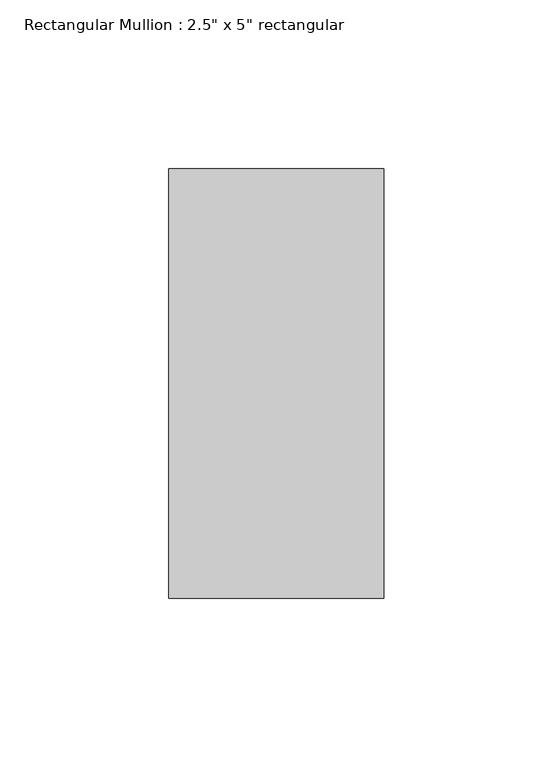
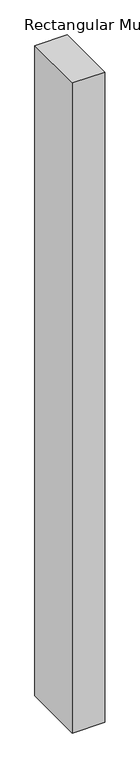
"""IFC4 building model written with IfcOpenShell, lengths in millimetres: member geometry."""

from ifc_helpers import new_model, si_unit, frame, origin, place, context, project, spatial, polyline, outline, extrude, source, transform, mapped, element, save


def member_a910906a(model_context):
    return source(origin(), model_context, "Body", "SweptSolid", [
        extrude(outline(polyline([(31.75, 63.5), (31.75, -63.5), (-31.75, -63.5), (-31.75, 63.5), (31.75, 63.5)])), frame((0.0, 0.0, -1349.975361), z_axis=(0.0, 0.0, 1.0), x_axis=(1.0, 0.0, 0.0)), (0.0, 0.0, 1.0), 1349.975361),
    ])


if __name__ == "__main__":
    model = new_model("IFC4")
    model_context = context("Model", 3, world=origin())
    ifc_project = project(units=[si_unit("LENGTHUNIT", "METRE", prefix="MILLI")], contexts=[model_context])
    site = spatial("IfcSite", under=ifc_project)
    building = spatial("IfcBuilding", under=site)
    placement = place(None, origin())
    member_shape = member_a910906a(model_context)
    element("IfcMember", 1, ObjectType="Rectangular Mullion : 2.5\" x 5\" rectangular", at=placement, inside=building, context=model_context, shape_type="MappedRepresentation", body=[
        mapped(member_shape, transform((0.0, 0.0, 0.0), x_axis=(1.0, 0.0, 0.0), y_axis=(0.0, 1.0, 0.0), z_axis=(0.0, 0.0, 1.0))),
    ])
    save(model, "model.ifc")

# Revit data of these elements
# Type "Rectangular Mullion : 2.5\" x 5\" rectangular"
#   built-in parameter 1007304 = 0.416667 (stored number, unit not read)
#   built-in parameter 1007301 = 0.104167 (stored number, unit not read)
#   built-in parameter 1007300 = 0.104167 (stored number, unit not read)
# Element 1 (IfcMember, "Rectangular Mullion : 2.5\" x 5\" rectangular")
#   Materials on its faces: "Aluminum"
# Materials
#   "Aluminum": class "Metal", colour RGB 247 247 247, transparency 0, Description = "Aluminum 6061", Cost = 0
